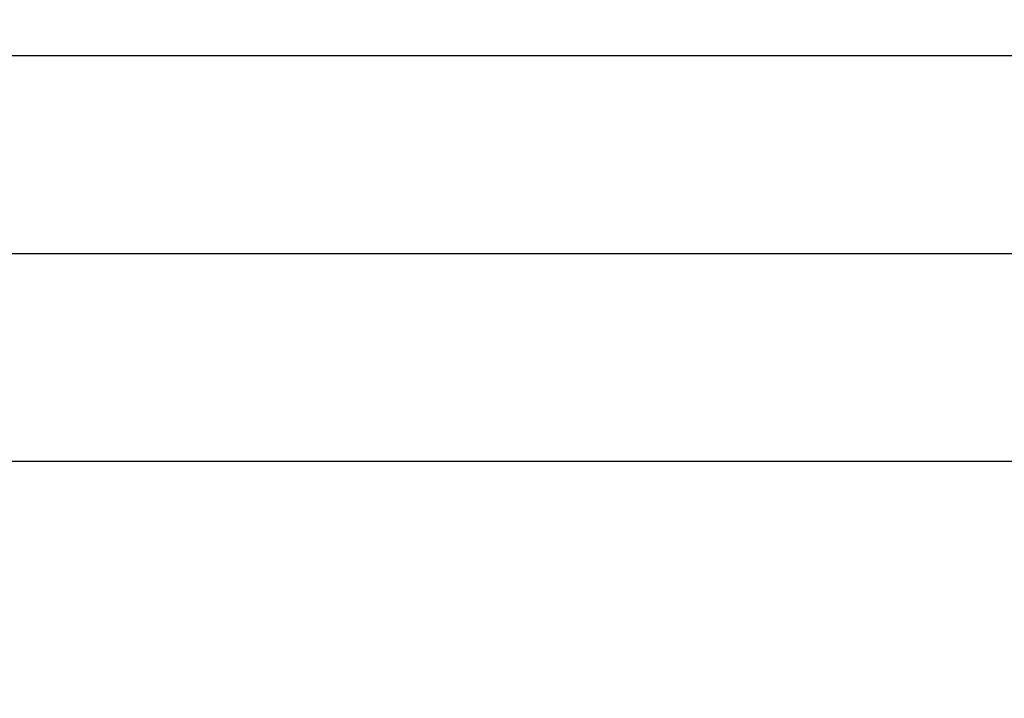
# Model space of a CAD drawing. Units: millimetres. Extents: x 7894 to 8038, y 6851 to 6951.
# Tile 28 of 49: x 7958.696 to 7968.188, y 6916.434 to 6922.974. Entities that reach past the tile are written whole.
import ezdxf

# ---------------------------------------------------------------- set-up
doc = ezdxf.new("R2010")
doc.units = ezdxf.units.MM
doc.layers.add('A-ANNO-DIMS', color=2, linetype='Continuous', lineweight=18)
doc.layers.add('A-FURN-SHLF', color=7, linetype='Continuous', lineweight=30)
doc.styles.get("Standard").update_dxf_attribs({"font": 'arial.ttf'})
doc.dimstyles.new('ISO-25', dxfattribs={"dimtxt": 1, "dimasz": 1, "dimexe": 1.25, "dimexo": 0.625, "dimtad": 1, "dimdec": 0, "dimlunit": 4, "dimtxsty": 'Standard', "dimcen": 2.5, "dimclrt": 1, "dimadec": 0, "dimazin": 0, "dimtfac": 1, "dimtdec": 0, "dimtmove": 0, "dimatfit": 3, "dimfxl": 1, "dimarcsym": 0})

# ---------------------------------------------------------------- blocks, each defined once
blk = doc.blocks.new('*D23')
at = {"layer": 'A-ANNO-DIMS', "color": 0, "lineweight": -2, "transparency": 16777216}
for p, q in [((7940.0888, 6907.098), (7940.0888, 6947.7928)), ((7971.9356, 6928.989), (7971.9356, 6947.7928)), ((7941.0888, 6946.5428), (7970.9356, 6946.5428))]:
    blk.add_line(p, q, dxfattribs=at)
at = {"layer": 'A-ANNO-DIMS', "color": 0, "transparency": 16777216}
for points in [[(7941.0888, 6946.7095), (7941.0888, 6946.3762), (7940.0888, 6946.5428)], [(7970.9356, 6946.7095), (7970.9356, 6946.3762), (7971.9356, 6946.5428)]]:
    blk.add_solid(points, dxfattribs=at)
at = {"layer": 'Defpoints', "color": 0, "transparency": 16777216}
for p in [(7971.9356, 6946.5428), (7971.9356, 6928.364), (7940.0888, 6906.473)]:
    blk.add_point(p, dxfattribs=at)
at = {"layer": 'A-ANNO-DIMS', "color": 1, "transparency": 16777216, "insert": (7956.0122, 6947.6784), "char_height": 1, "attachment_point": 5}
blk.add_mtext('2\'-8"', dxfattribs=at)
blk = doc.blocks.new('*D26')
at = {"layer": 'A-ANNO-DIMS', "color": 0, "lineweight": -2, "transparency": 16777216}
for p, q in [((7950.9654, 6918.7198), (7975.2272, 6918.7198)), ((7973.9772, 6917.7198), (7973.9772, 6907.4734)), ((7964.9658, 6906.4734), (7975.2272, 6906.4734))]:
    blk.add_line(p, q, dxfattribs=at)
at = {"layer": 'A-ANNO-DIMS', "color": 0, "transparency": 16777216}
for points in [[(7973.8105, 6917.7198), (7974.1439, 6917.7198), (7973.9772, 6918.7198)], [(7973.8105, 6907.4734), (7974.1439, 6907.4734), (7973.9772, 6906.4734)]]:
    blk.add_solid(points, dxfattribs=at)
at = {"layer": 'Defpoints', "color": 0, "transparency": 16777216}
for p in [(7950.3404, 6918.7198), (7964.3408, 6906.4734), (7973.9772, 6906.4734)]:
    blk.add_point(p, dxfattribs=at)
at = {"layer": 'A-ANNO-DIMS', "color": 1, "transparency": 16777216, "insert": (7972.8416, 6912.5966), "char_height": 1, "attachment_point": 5, "rotation": 90}
blk.add_mtext('1\'-0"', dxfattribs=at)
blk = doc.blocks.new('*D27')
at = {"layer": 'A-ANNO-DIMS', "color": 0, "lineweight": -2, "transparency": 16777216}
for p, q in [((7971.8421, 6922.6283), (7975.2272, 6922.6283)), ((7973.9772, 6921.6283), (7973.9772, 6919.7198)), ((7950.9654, 6918.7198), (7975.2272, 6918.7198))]:
    blk.add_line(p, q, dxfattribs=at)
at = {"layer": 'A-ANNO-DIMS', "color": 0, "transparency": 16777216}
for points in [[(7973.8105, 6921.6283), (7974.1439, 6921.6283), (7973.9772, 6922.6283)], [(7973.8105, 6919.7198), (7974.1439, 6919.7198), (7973.9772, 6918.7198)]]:
    blk.add_solid(points, dxfattribs=at)
at = {"layer": 'Defpoints', "color": 0, "transparency": 16777216}
for p in [(7971.2171, 6922.6283), (7950.3404, 6918.7198), (7973.9772, 6918.7198)]:
    blk.add_point(p, dxfattribs=at)
at = {"layer": 'A-ANNO-DIMS', "color": 1, "transparency": 16777216, "insert": (7972.8416, 6920.6741), "char_height": 1, "attachment_point": 5, "rotation": 90}
blk.add_mtext('0\'-4"', dxfattribs=at)
blk = doc.blocks.new('*D28')
at = {"layer": 'A-ANNO-DIMS', "color": 0, "lineweight": -2, "transparency": 16777216}
for p, q in [((7960.8854, 6936.8804), (7975.2272, 6936.8804)), ((7973.9772, 6935.8804), (7973.9772, 6923.6283)), ((7971.8421, 6922.6283), (7975.2272, 6922.6283))]:
    blk.add_line(p, q, dxfattribs=at)
at = {"layer": 'A-ANNO-DIMS', "color": 0, "transparency": 16777216}
for points in [[(7973.8105, 6935.8804), (7974.1439, 6935.8804), (7973.9772, 6936.8804)], [(7973.8105, 6923.6283), (7974.1439, 6923.6283), (7973.9772, 6922.6283)]]:
    blk.add_solid(points, dxfattribs=at)
at = {"layer": 'Defpoints', "color": 0, "transparency": 16777216}
for p in [(7960.2604, 6936.8804), (7971.2171, 6922.6283), (7973.9772, 6922.6283)]:
    blk.add_point(p, dxfattribs=at)
at = {"layer": 'A-ANNO-DIMS', "color": 1, "transparency": 16777216, "insert": (7972.8351, 6929.7543), "char_height": 1, "attachment_point": 5, "rotation": 90}
blk.add_mtext('1\'-2 1/2"', dxfattribs=at)
blk = doc.blocks.new('*D31')
at = {"layer": 'A-ANNO-DIMS', "color": 0, "lineweight": -2, "transparency": 16777216}
for p, q in [((7973.9772, 6921.7198), (7973.9772, 6926.628)), ((7949.8107, 6920.7198), (7975.2272, 6920.7198)), ((7973.9772, 6918.7198), (7973.9772, 6920.7198)), ((7950.9654, 6918.7198), (7975.2272, 6918.7198)), ((7973.9772, 6917.7198), (7973.9772, 6916.7198))]:
    blk.add_line(p, q, dxfattribs=at)
at = {"layer": 'A-ANNO-DIMS', "color": 0, "transparency": 16777216}
for points in [[(7973.8105, 6921.7198), (7974.1439, 6921.7198), (7973.9772, 6920.7198)], [(7973.8105, 6917.7198), (7974.1439, 6917.7198), (7973.9772, 6918.7198)]]:
    blk.add_solid(points, dxfattribs=at)
at = {"layer": 'Defpoints', "color": 0, "transparency": 16777216}
for p in [(7949.1857, 6920.7198), (7973.9772, 6920.7198), (7950.3404, 6918.7198)]:
    blk.add_point(p, dxfattribs=at)
at = {"layer": 'A-ANNO-DIMS', "color": 1, "transparency": 16777216, "insert": (7972.8416, 6924.6739), "char_height": 1, "attachment_point": 5, "rotation": 90}
blk.add_mtext('0\'-2"', dxfattribs=at)
blk = doc.blocks.new('*D34')
at = {"layer": 'A-ANNO-DIMS', "color": 0, "lineweight": -2, "transparency": 16777216}
for p, q in [((7971.2171, 6922.0033), (7971.2171, 6903.2865)), ((7964.3408, 6905.8484), (7964.3408, 6903.2865)), ((7965.3408, 6904.5365), (7970.2171, 6904.5365))]:
    blk.add_line(p, q, dxfattribs=at)
at = {"layer": 'A-ANNO-DIMS', "color": 0, "transparency": 16777216}
for points in [[(7965.3408, 6904.7032), (7965.3408, 6904.3699), (7964.3408, 6904.5365)], [(7970.2171, 6904.7032), (7970.2171, 6904.3699), (7971.2171, 6904.5365)]]:
    blk.add_solid(points, dxfattribs=at)
at = {"layer": 'Defpoints', "color": 0, "transparency": 16777216}
for p in [(7971.2171, 6922.6283), (7964.3408, 6906.4734), (7971.2171, 6904.5365)]:
    blk.add_point(p, dxfattribs=at)
at = {"layer": 'A-ANNO-DIMS', "color": 1, "transparency": 16777216, "insert": (7967.779, 6905.6721), "char_height": 1, "attachment_point": 5}
blk.add_mtext('0\'-7"', dxfattribs=at)

msp = doc.modelspace()

# ---------------------------------------------------------------- linework, layer by layer
at = {"layer": 'A-FURN-SHLF'}
msp.add_line((7953.9136, 6922.6283, -7), (7971.2171, 6922.6283, -7), dxfattribs=at)

# ---------------------------------------------------------------- dimensions: what is measured, and where the dimension line sits
at = {"layer": 'A-ANNO-DIMS'}
for base, p1, p2, picture, middle in [((7971.9356, 6946.5428), (7940.0888, 6906.473), (7971.9356, 6928.364), '*D23', (7956.0122, 6947.6784)), ((7971.2171, 6904.5365), (7964.3408, 6906.4734), (7971.2171, 6922.6283), '*D34', (7967.779, 6905.6721))]:
    dim = msp.add_linear_dim(base=base, p1=p1, p2=p2, dimstyle='ISO-25', override={"dimdec": 1, "dimlfac": 1, "dimrnd": 0, "dimzin": 1, "dimdsep": 46, "dimlunit": 4, "dimfrac": 2}, dxfattribs=at)
    dim.commit()
    dim.dimension.update_dxf_attribs({"geometry": picture, "text_midpoint": middle})
for base, p1, p2, picture, middle in [((7973.9772, 6922.6283), (7960.2604, 6936.8804), (7971.2171, 6922.6283), '*D28', (7972.8351, 6929.7543)), ((7973.9772, 6920.7198), (7950.3404, 6918.7198), (7949.1857, 6920.7198), '*D31', (7972.8416, 6924.6739)), ((7973.9772, 6918.7198), (7971.2171, 6922.6283), (7950.3404, 6918.7198), '*D27', (7972.8416, 6920.6741)), ((7973.9772, 6906.4734), (7950.3404, 6918.7198), (7964.3408, 6906.4734), '*D26', (7972.8416, 6912.5966))]:
    dim = msp.add_linear_dim(base=base, p1=p1, p2=p2, angle=90, dimstyle='ISO-25', override={"dimdec": 1, "dimlfac": 1, "dimrnd": 0, "dimzin": 1, "dimdsep": 46, "dimlunit": 4, "dimfrac": 2}, dxfattribs=at)
    dim.commit()
    dim.dimension.update_dxf_attribs({"geometry": picture, "text_midpoint": middle})

doc.saveas('drawing.dxf')
